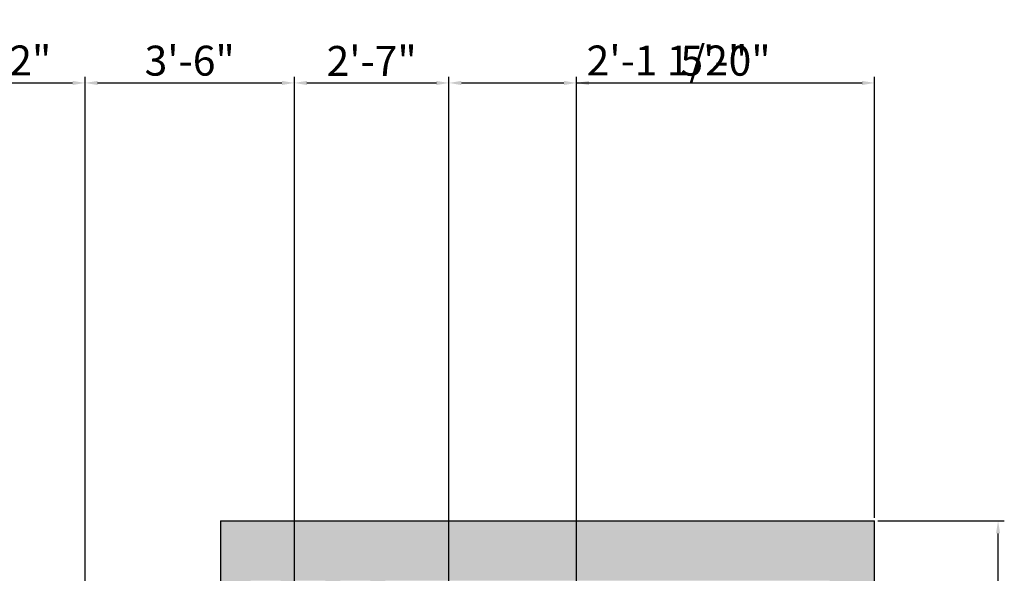
# Model space of a CAD drawing. Units: millimetres. Extents: x 4237 to 5109, y 21391 to 22486.
# Tile 5 of 17: x 4911 to 5109, y 21798 to 21909. Entities that reach past the tile are written whole.
import ezdxf

# ---------------------------------------------------------------- set-up
doc = ezdxf.new("R2010")
doc.units = ezdxf.units.MM
for name, color, linetype, lineweight in [('A-ANNO-DIMS', 2, 'Continuous', 18), ('A-ELEV', 7, 'Continuous', 25), ('A-ELEV-PATT', 252, 'Continuous', 13)]:
    doc.layers.add(name, color=color, linetype=linetype, lineweight=lineweight)
doc.styles.get("Standard").update_dxf_attribs({"font": 'arial.ttf'})
doc.dimstyles.new('ISO-25', dxfattribs={"dimtxt": 6, "dimasz": 2.5, "dimexe": 1.25, "dimexo": 0.625, "dimtad": 1, "dimdec": 1, "dimlunit": 4, "dimtxsty": 'Standard', "dimcen": 2.5, "dimadec": 0, "dimazin": 0, "dimtfac": 1, "dimtdec": 1, "dimtmove": 0, "dimatfit": 3, "dimfxl": 1, "dimarcsym": 0})

# ---------------------------------------------------------------- blocks, each defined once
blk = doc.blocks.new('*D130')
at = {"layer": 'A-ANNO-DIMS', "color": 0, "lineweight": -2, "transparency": 16777216}
for p, q in [((4878.54, 21688.54), (4878.54, 21897.84)), ((4881.04, 21896.59), (4921.78, 21896.59)), ((4924.28, 21686.68), (4924.28, 21897.84))]:
    blk.add_line(p, q, dxfattribs=at)
at = {"layer": 'A-ANNO-DIMS', "color": 0, "transparency": 16777216}
for points in [[(4881.04, 21897), (4881.04, 21896.17), (4878.54, 21896.59)], [(4921.78, 21897), (4921.78, 21896.17), (4924.28, 21896.59)]]:
    blk.add_solid(points, dxfattribs=at)
at = {"layer": 'Defpoints', "color": 0, "transparency": 16777216}
for p in [(4924.28, 21896.59), (4878.54, 21687.91), (4924.28, 21686.05)]:
    blk.add_point(p, dxfattribs=at)
at = {"layer": 'A-ANNO-DIMS', "color": 0, "transparency": 16777216, "insert": (4901.41, 21900.32), "char_height": 6, "attachment_point": 5}
blk.add_mtext('3\'-9 1/2"', dxfattribs=at)
blk = doc.blocks.new('*D131')
at = {"layer": 'A-ANNO-DIMS', "color": 0, "lineweight": -2, "transparency": 16777216}
for p, q in [((4924.28, 21686.68), (4924.28, 21897.84)), ((4926.78, 21896.59), (4963.73, 21896.59)), ((4966.23, 21686.68), (4966.23, 21897.84))]:
    blk.add_line(p, q, dxfattribs=at)
at = {"layer": 'A-ANNO-DIMS', "color": 0, "transparency": 16777216}
for points in [[(4926.78, 21897), (4926.78, 21896.17), (4924.28, 21896.59)], [(4963.73, 21897), (4963.73, 21896.17), (4966.23, 21896.59)]]:
    blk.add_solid(points, dxfattribs=at)
at = {"layer": 'Defpoints', "color": 0, "transparency": 16777216}
for p in [(4966.23, 21896.59), (4924.28, 21686.05), (4966.23, 21686.05)]:
    blk.add_point(p, dxfattribs=at)
at = {"layer": 'A-ANNO-DIMS', "color": 0, "transparency": 16777216, "insert": (4945.25, 21900.28), "char_height": 6, "attachment_point": 5}
blk.add_mtext('3\'-6"', dxfattribs=at)
blk = doc.blocks.new('*D132')
at = {"layer": 'A-ANNO-DIMS', "color": 0, "lineweight": -2, "transparency": 16777216}
for p, q in [((4966.23, 21686.68), (4966.23, 21897.84)), ((4968.73, 21896.59), (4994.7, 21896.59)), ((4997.2, 21689.78), (4997.2, 21897.84))]:
    blk.add_line(p, q, dxfattribs=at)
at = {"layer": 'A-ANNO-DIMS', "color": 0, "transparency": 16777216}
for points in [[(4968.73, 21897), (4968.73, 21896.17), (4966.23, 21896.59)], [(4994.7, 21897), (4994.7, 21896.17), (4997.2, 21896.59)]]:
    blk.add_solid(points, dxfattribs=at)
at = {"layer": 'Defpoints', "color": 0, "transparency": 16777216}
for p in [(4997.2, 21896.59), (4997.2, 21689.16), (4966.23, 21686.05)]:
    blk.add_point(p, dxfattribs=at)
at = {"layer": 'A-ANNO-DIMS', "color": 0, "transparency": 16777216, "insert": (4981.72, 21900.22), "char_height": 6, "attachment_point": 5}
blk.add_mtext('2\'-7"', dxfattribs=at)
blk = doc.blocks.new('*D133')
at = {"layer": 'A-ANNO-DIMS', "color": 0, "lineweight": -2, "transparency": 16777216}
for p, q in [((4997.2, 21689.78), (4997.2, 21897.84)), ((4999.7, 21896.59), (5020.26, 21896.59)), ((5022.76, 21689.78), (5022.76, 21897.84)), ((5022.76, 21896.59), (5056.55, 21896.59))]:
    blk.add_line(p, q, dxfattribs=at)
at = {"layer": 'A-ANNO-DIMS', "color": 0, "transparency": 16777216}
for points in [[(4999.7, 21897), (4999.7, 21896.17), (4997.2, 21896.59)], [(5020.26, 21897), (5020.26, 21896.17), (5022.76, 21896.59)]]:
    blk.add_solid(points, dxfattribs=at)
at = {"layer": 'Defpoints', "color": 0, "transparency": 16777216}
for p in [(5022.76, 21896.59), (4997.2, 21689.16), (5022.76, 21689.16)]:
    blk.add_point(p, dxfattribs=at)
at = {"layer": 'A-ANNO-DIMS', "color": 0, "transparency": 16777216, "insert": (5040.91, 21900.31), "char_height": 6, "attachment_point": 5}
blk.add_mtext('2\'-1 1/2"', dxfattribs=at)
blk = doc.blocks.new('*D134')
at = {"layer": 'A-ANNO-DIMS', "color": 0, "lineweight": -2, "transparency": 16777216}
for p, q in [((5022.76, 21689.78), (5022.76, 21897.84)), ((5025.26, 21896.59), (5080.03, 21896.59)), ((5082.53, 21809.46), (5082.53, 21897.84))]:
    blk.add_line(p, q, dxfattribs=at)
at = {"layer": 'A-ANNO-DIMS', "color": 0, "transparency": 16777216}
for points in [[(5025.26, 21897), (5025.26, 21896.17), (5022.76, 21896.59)], [(5080.03, 21897), (5080.03, 21896.17), (5082.53, 21896.59)]]:
    blk.add_solid(points, dxfattribs=at)
at = {"layer": 'Defpoints', "color": 0, "transparency": 16777216}
for p in [(5082.53, 21896.59), (5082.53, 21808.84), (5022.76, 21689.16)]:
    blk.add_point(p, dxfattribs=at)
at = {"layer": 'A-ANNO-DIMS', "color": 0, "transparency": 16777216, "insert": (5052.65, 21900.27), "char_height": 6, "attachment_point": 5}
blk.add_mtext('5\'-0"', dxfattribs=at)
blk = doc.blocks.new('*D137')
at = {"layer": 'A-ANNO-DIMS', "color": 0, "lineweight": -2, "transparency": 16777216}
for p, q in [((5083.15, 21808.84), (5108.53, 21808.84)), ((5107.28, 21730.34), (5107.28, 21806.34)), ((5074.15, 21727.84), (5108.53, 21727.84))]:
    blk.add_line(p, q, dxfattribs=at)
at = {"layer": 'A-ANNO-DIMS', "color": 0, "transparency": 16777216}
for points in [[(5106.86, 21806.34), (5107.69, 21806.34), (5107.28, 21808.84)], [(5106.86, 21730.34), (5107.69, 21730.34), (5107.28, 21727.84)]]:
    blk.add_solid(points, dxfattribs=at)
at = {"layer": 'Defpoints', "color": 0, "transparency": 16777216}
for p in [(5082.53, 21808.84), (5107.28, 21808.84), (5073.53, 21727.84)]:
    blk.add_point(p, dxfattribs=at)
at = {"layer": 'A-ANNO-DIMS', "color": 0, "transparency": 16777216, "insert": (5103.59, 21768.34), "char_height": 6, "attachment_point": 5, "rotation": 90}
blk.add_mtext('6\'-9"', dxfattribs=at)

msp = doc.modelspace()

# ---------------------------------------------------------------- hatches: boundary and pattern name
at = {"layer": 'A-ELEV-PATT'}
h = msp.add_hatch(color=256, dxfattribs=at)
h.dxf.hatch_style = 1
h.paths.add_polyline_path([(4957.45, 21796.84), (4963.45, 21796.84), (4963.45, 21727.84), (4966.45, 21727.84), (4966.45, 21796.84), (4972.45, 21796.84), (4972.45, 21727.84), (4975.45, 21727.84), (4975.45, 21796.84), (4981.45, 21796.84), (4981.45, 21727.84), (4984.45, 21727.84), (4984.45, 21796.84), (5073.53, 21796.84), (5073.53, 21557.84), (5082.53, 21557.84), (5082.53, 21808.84), (4951.45, 21808.84), (4951.45, 21727.84), (4957.45, 21727.84)])

# ---------------------------------------------------------------- linework, layer by layer
at = {"layer": 'A-ELEV'}
for p, q in [((4951.45, 21808.84), (5082.53, 21808.84)), ((4951.45, 21808.84), (4951.45, 21727.84)), ((5082.53, 21425.84), (5082.53, 21808.84))]:
    msp.add_line(p, q, dxfattribs=at)

# ---------------------------------------------------------------- dimensions: what is measured, and where the dimension line sits
at = {"layer": 'A-ANNO-DIMS'}
for base, p1, p2, picture, middle in [((4924.28, 21896.59), (4878.54, 21687.91), (4924.28, 21686.05), '*D130', (4901.41, 21900.32)), ((5022.76, 21896.59), (4997.2, 21689.16), (5022.76, 21689.16), '*D133', (5040.91, 21900.31)), ((4966.2267, 21896.586), (4924.2801, 21686.0515), (4966.2267, 21686.0515), '*D131', (4945.2534, 21900.2765)), ((4997.2, 21896.59), (4966.23, 21686.05), (4997.2, 21689.16), '*D132', (4981.72, 21900.22)), ((5082.53, 21896.59), (5022.76, 21689.16), (5082.53, 21808.84), '*D134', (5052.65, 21900.27))]:
    dim = msp.add_linear_dim(base=base, p1=p1, p2=p2, dimstyle='ISO-25', override={"dimdec": 1, "dimlfac": 1, "dimrnd": 0, "dimzin": 1, "dimdsep": 46, "dimlunit": 4, "dimfrac": 2}, dxfattribs=at)
    dim.commit()
    dim.dimension.update_dxf_attribs({"geometry": picture, "text_midpoint": middle})
dim = msp.add_linear_dim(base=(5107.28, 21808.84), p1=(5073.53, 21727.84), p2=(5082.53, 21808.84), angle=90, dimstyle='ISO-25', override={"dimdec": 1, "dimlfac": 1, "dimrnd": 0, "dimzin": 1, "dimdsep": 46, "dimlunit": 4, "dimfrac": 2}, dxfattribs=at)
dim.commit()
dim.dimension.update_dxf_attribs({"geometry": '*D137', "text_midpoint": (5103.59, 21768.34)})

doc.saveas('drawing.dxf')
